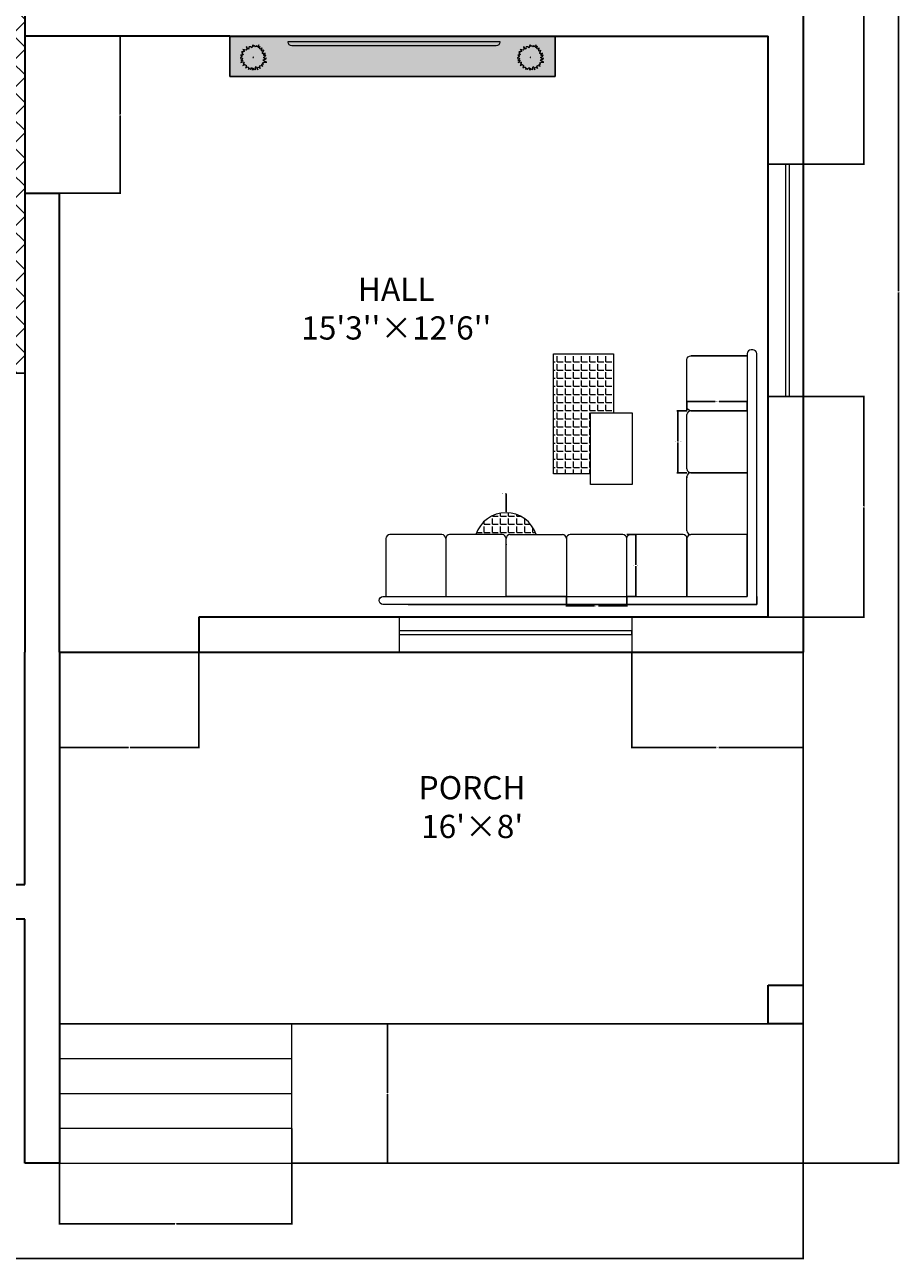
# Model space of a CAD drawing. Units: inches. Extents: x 1315 to 1802, y 1702 to 2202.
# Tile 3 of 4: x 1577 to 1802, y 1702 to 2021. Entities that reach past the tile are written whole.
import ezdxf

# ---------------------------------------------------------------- set-up
doc = ezdxf.new("R2010")
doc.units = ezdxf.units.IN
for name, color, linetype, lineweight in [('A-ANNO-DIMS', 2, 'Continuous', 18), ('A-AREA-IDEN', 3, 'Continuous', 18), ('A-CASE', 7, 'Continuous', 25), ('A-CASE-PATT', 246, 'Continuous', 13), ('A-COLS', 7, 'Continuous', 35), ('A-EQPM', 3, 'Continuous', 18), ('A-FLOR', 7, 'Continuous', 25), ('A-FLOR-PATT', 254, 'Continuous', 13), ('A-FLOR-STRS', 7, 'Continuous', 18), ('A-FURN', 8, 'Continuous', 18), ('A-FURN-PATT', 9, 'Continuous', 13), ('A-GLAZ', 4, 'Continuous', 18), ('A-WALL', 7, 'Continuous', 35)]:
    doc.layers.add(name, color=color, linetype=linetype, lineweight=lineweight)
doc.styles.get("Standard").update_dxf_attribs({"font": 'times.ttf'})
doc.dimstyles.get("Standard").update_dxf_attribs({"dimtxt": 0.18, "dimasz": 0.18, "dimexe": 0.18, "dimexo": 0.0625, "dimgap": 0.09, "dimtad": 0, "dimtih": 1, "dimtoh": 1, "dimdec": 4, "dimzin": 0, "dimdsep": 46, "dimtxsty": 'Standard', "dimcen": 0.09, "dimadec": 0, "dimazin": 0, "dimtfac": 1, "dimtdec": 4, "dimtofl": 0, "dimtmove": 0, "dimatfit": 3, "dimfxl": 1, "dimtolj": 1, "dimtzin": 0, "dimarcsym": 0})

# ---------------------------------------------------------------- blocks, each defined once
blk = doc.blocks.new('*U2')
for points in [[(0, 60.64), (-3.051, 56.238), (-4.196, 52.815), (-5.34, 47.925), (-6.103, 45.969), (-11.062, 50.859), (-18.691, 52.326), (-20.98, 47.436), (-20.217, 43.524), (-20.598, 39.611), (-25.939, 43.035), (-27.846, 49.392), (-33.186, 52.326), (-30.516, 47.436), (-31.279, 43.035), (-30.135, 38.144), (-33.568, 35.21), (-40.815, 36.677), (-49.208, 38.144), (-46.919, 36.677), (-42.341, 31.787), (-42.341, 28.364), (-46.537, 27.386), (-55.692, 27.386), (-49.97, 22.006), (-54.548, 21.028), (-46.156, 14.671), (-51.496, 11.248), (-59.888, 11.248), (-55.692, 8.803), (-53.785, 5.38), (-57.218, 3.423), (-60.651, -1.467), (-61.033, -4.89), (-59.125, -3.423), (-54.548, -1.467), (-51.496, -4.401), (-53.022, -10.269), (-59.125, -15.16), (-49.208, -13.204), (-58.362, -24.451), (-48.445, -21.028), (-43.486, -22.495), (-43.104, -25.918), (-47.3, -31.298), (-43.104, -30.32), (-48.445, -39.611), (-38.527, -31.787), (-40.815, -36.188), (-32.423, -37.166), (-33.568, -43.523), (-35.475, -49.392), (-28.609, -44.99), (-23.65, -46.457), (-22.124, -51.837), (-21.743, -57.705), (-19.073, -52.326), (-15.639, -51.837), (-12.588, -58.683), (-11.062, -54.771), (-6.866, -49.392), (-6.866, -53.304), (-4.959, -48.414), (-1.907, -61.617), (-1.144, -51.348), (4.578, -59.172), (5.341, -54.282), (9.918, -56.727), (12.207, -60.639), (12.97, -47.925), (14.877, -44.501), (17.547, -47.436), (19.455, -52.815), (22.888, -60.639), (21.743, -49.392), (23.65, -46.457), (29.754, -47.925), (35.094, -52.326), (37.001, -53.793), (33.187, -46.457), (32.042, -41.567), (35.094, -39.122), (43.868, -40.589), (47.682, -42.056), (43.105, -36.188), (43.105, -33.743), (46.538, -31.298), (50.352, -32.765), (46.919, -26.407), (55.693, -22.495), (60.652, -22.984), (66.374, -22.006), (59.889, -20.05), (54.167, -18.094), (51.878, -15.649), (49.589, -12.225), (51.497, -10.269), (57.981, -9.78), (63.322, -7.335), (64.466, -2.934)], [(64.848, -2.934), (59.507, -5.379), (56.456, -4.401), (51.878, -2.445), (52.26, 0.978), (55.311, 3.912), (59.889, 5.869), (62.94, 11.248), (58.363, 10.27), (54.548, 10.27), (51.115, 11.248), (53.785, 15.649), (57.981, 18.094), (60.652, 19.561), (56.074, 19.561), (51.115, 17.605), (46.538, 19.072), (46.156, 22.496), (49.589, 27.386), (52.26, 34.721), (49.589, 33.743), (44.249, 30.32), (41.197, 32.276), (41.579, 37.655), (43.868, 42.546), (43.105, 46.947), (40.053, 44.013), (36.238, 40.589), (33.568, 42.057), (33.95, 45.969), (35.476, 52.815), (31.28, 49.392), (26.702, 46.947), (28.228, 50.859), (28.609, 61.129), (24.795, 54.282), (18.692, 50.859), (17.929, 57.706), (12.97, 50.859), (7.248, 57.706), (5.341, 53.304), (0, 60.64)]]:
    blk.add_lwpolyline(points)
blk.add_lwpolyline([(0.382, 1.956), (0, 0), (1.907, 0.489), (2.289, 1.467)], close=True)
blk = doc.blocks.new('SEFVFT')
for p, q in [((1768.59, 1985.26), (1777.59, 1985.26)), ((1768.59, 1925.26), (1768.59, 1985.26)), ((1768.59, 1985.26), (1773.09, 1985.26)), ((1773.09, 1985.26), (1773.09, 1925.26)), ((1774.09, 1925.26), (1774.09, 1985.26)), ((1777.59, 1985.26), (1777.59, 1925.26)), ((1777.59, 1925.26), (1768.59, 1925.26)), ((1773.09, 1925.26), (1774.09, 1925.26))]:
    blk.add_line(p, q)
blk = doc.blocks.new('SOFA-SEAT')
for p, q in [((14.58, 16), (1, 16)), ((0, 15), (0, 0)), ((15.58, 0), (15.58, 15)), ((0, 0), (15.58, 0))]:
    blk.add_line(p, q)
for centre, start, end in [((1, 15), 90, 180), ((14.58, 15), 0, 90)]:
    blk.add_arc(centre, 1, start, end)
blk = doc.blocks.new('SOFA-RETURN-SEAT')
for p, q in [((1, 16), (15.58, 16)), ((15.58, 16), (15.58, 0)), ((0, 1), (0, 15)), ((15.58, 0), (1, 0))]:
    blk.add_line(p, q)
for centre, start, end in [((1, 15), 90, 180), ((1, 1), 180, 270)]:
    blk.add_arc(centre, 1, start, end)
blk = doc.blocks.new('*D24')
at = {"layer": 'A-ANNO-DIMS', "color": 0, "lineweight": -2, "transparency": 16777216}
for p, q in [((1732.1, 1889.55), (1734.62, 1889.55)), ((1734.44, 1889.37), (1734.44, 1881.73)), ((1734.44, 1873.73), (1734.44, 1881.37)), ((1732.1, 1873.55), (1734.62, 1873.55))]:
    blk.add_line(p, q, dxfattribs=at)
at = {"layer": 'A-ANNO-DIMS', "color": 0, "transparency": 16777216}
for points in [[(1734.41, 1889.37), (1734.47, 1889.37), (1734.44, 1889.55)], [(1734.41, 1873.73), (1734.47, 1873.73), (1734.44, 1873.55)]]:
    blk.add_solid(points, dxfattribs=at)
at = {"layer": 'Defpoints', "color": 0, "transparency": 16777216}
for p in [(1732.04, 1889.55), (1734.44, 1889.55), (1732.04, 1873.55)]:
    blk.add_point(p, dxfattribs=at)
at = {"layer": 'A-ANNO-DIMS', "color": 0, "transparency": 16777216, "insert": (1734.44, 1881.55), "char_height": 0.18, "attachment_point": 5}
blk.add_mtext('\\A1;SEAT 16 TYP.', dxfattribs=at)
blk = doc.blocks.new('*D25')
at = {"layer": 'A-ANNO-DIMS', "color": 0, "lineweight": -2, "transparency": 16777216}
for p, q in [((1716.46, 1873.49), (1716.46, 1870.97)), ((1732.04, 1873.49), (1732.04, 1870.97)), ((1716.64, 1871.15), (1723.74, 1871.15)), ((1731.86, 1871.15), (1724.77, 1871.15))]:
    blk.add_line(p, q, dxfattribs=at)
at = {"layer": 'A-ANNO-DIMS', "color": 0, "transparency": 16777216}
for points in [[(1716.64, 1871.18), (1716.64, 1871.12), (1716.46, 1871.15)], [(1731.86, 1871.18), (1731.86, 1871.12), (1732.04, 1871.15)]]:
    blk.add_solid(points, dxfattribs=at)
at = {"layer": 'Defpoints', "color": 0, "transparency": 16777216}
for p in [(1716.46, 1873.55), (1732.04, 1873.55), (1732.04, 1871.15)]:
    blk.add_point(p, dxfattribs=at)
at = {"layer": 'A-ANNO-DIMS', "color": 0, "transparency": 16777216, "insert": (1724.25, 1871.15), "char_height": 0.18, "attachment_point": 5}
blk.add_mtext('\\A1;16 TYP.', dxfattribs=at)
blk = doc.blocks.new('*D26')
at = {"layer": 'A-ANNO-DIMS', "color": 0, "lineweight": -2, "transparency": 16777216}
for p, q in [((1747.55, 1921.54), (1745.03, 1921.54)), ((1745.21, 1921.36), (1745.21, 1913.73)), ((1745.21, 1905.73), (1745.21, 1913.36)), ((1747.55, 1905.55), (1745.03, 1905.55))]:
    blk.add_line(p, q, dxfattribs=at)
at = {"layer": 'A-ANNO-DIMS', "color": 0, "transparency": 16777216}
for points in [[(1745.18, 1921.36), (1745.24, 1921.36), (1745.21, 1921.54)], [(1745.18, 1905.73), (1745.24, 1905.73), (1745.21, 1905.55)]]:
    blk.add_solid(points, dxfattribs=at)
at = {"layer": 'Defpoints', "color": 0, "transparency": 16777216}
for p in [(1745.21, 1921.54), (1747.61, 1921.54), (1747.61, 1905.55)]:
    blk.add_point(p, dxfattribs=at)
at = {"layer": 'A-ANNO-DIMS', "color": 0, "transparency": 16777216, "insert": (1745.21, 1913.55), "char_height": 0.18, "attachment_point": 5}
blk.add_mtext('\\A1;RETURN SEAT 16 TYP.', dxfattribs=at)
blk = doc.blocks.new('*D27')
at = {"layer": 'A-ANNO-DIMS', "color": 0, "lineweight": -2, "transparency": 16777216}
for p, q in [((1747.61, 1921.61), (1747.61, 1924.12)), ((1747.79, 1923.94), (1754.89, 1923.94)), ((1763.01, 1923.94), (1755.92, 1923.94)), ((1763.19, 1921.61), (1763.19, 1924.12))]:
    blk.add_line(p, q, dxfattribs=at)
at = {"layer": 'A-ANNO-DIMS', "color": 0, "transparency": 16777216}
for points in [[(1747.79, 1923.97), (1747.79, 1923.91), (1747.61, 1923.94)], [(1763.01, 1923.97), (1763.01, 1923.91), (1763.19, 1923.94)]]:
    blk.add_solid(points, dxfattribs=at)
at = {"layer": 'Defpoints', "color": 0, "transparency": 16777216}
for p in [(1763.19, 1923.94), (1747.61, 1921.54), (1763.19, 1921.54)]:
    blk.add_point(p, dxfattribs=at)
at = {"layer": 'A-ANNO-DIMS', "color": 0, "transparency": 16777216, "insert": (1755.4, 1923.94), "char_height": 0.18, "attachment_point": 5}
blk.add_mtext('\\A1;16 TYP.', dxfattribs=at)
blk = doc.blocks.new('*D28')
at = {"layer": 'A-ANNO-DIMS', "color": 0, "lineweight": -2, "transparency": 16777216}
for p, q in [((1339.59, 1931.18), (1339.59, 1702.41)), ((1777.59, 1763.18), (1777.59, 1702.41)), ((1339.77, 1702.59), (1558.31, 1702.59)), ((1777.41, 1702.59), (1558.87, 1702.59))]:
    blk.add_line(p, q, dxfattribs=at)
at = {"layer": 'A-ANNO-DIMS', "color": 0, "transparency": 16777216}
for points in [[(1339.77, 1702.62), (1339.77, 1702.56), (1339.59, 1702.59)], [(1777.41, 1702.62), (1777.41, 1702.56), (1777.59, 1702.59)]]:
    blk.add_solid(points, dxfattribs=at)
at = {"layer": 'Defpoints', "color": 0, "transparency": 16777216}
for p in [(1339.59, 1931.24), (1777.59, 1763.24), (1777.59, 1702.59)]:
    blk.add_point(p, dxfattribs=at)
at = {"layer": 'A-ANNO-DIMS', "color": 0, "transparency": 16777216, "insert": (1558.59, 1702.59), "char_height": 0.18, "attachment_point": 5}
blk.add_mtext('\\A1;438', dxfattribs=at)
blk = doc.blocks.new('*D29')
at = {"layer": 'A-ANNO-DIMS', "color": 0, "lineweight": -2, "transparency": 16777216}
for p, q in [((1777.65, 2177.24), (1802.42, 2177.24)), ((1802.24, 2177.06), (1802.24, 1952.42)), ((1802.24, 1727.42), (1802.24, 1952.06)), ((1645.65, 1727.24), (1802.42, 1727.24))]:
    blk.add_line(p, q, dxfattribs=at)
at = {"layer": 'A-ANNO-DIMS', "color": 0, "transparency": 16777216}
for points in [[(1802.21, 2177.06), (1802.27, 2177.06), (1802.24, 2177.24)], [(1802.21, 1727.42), (1802.27, 1727.42), (1802.24, 1727.24)]]:
    blk.add_solid(points, dxfattribs=at)
at = {"layer": 'Defpoints', "color": 0, "transparency": 16777216}
for p in [(1777.59, 2177.24), (1802.24, 2177.24), (1645.59, 1727.24)]:
    blk.add_point(p, dxfattribs=at)
at = {"layer": 'A-ANNO-DIMS', "color": 0, "transparency": 16777216, "insert": (1802.24, 1952.24), "char_height": 0.18, "attachment_point": 5}
blk.add_mtext('\\A1;450', dxfattribs=at)
blk = doc.blocks.new('*D42')
at = {"layer": 'A-ANNO-DIMS', "color": 0, "lineweight": -2, "transparency": 16777216}
for p, q in [((1768.65, 2072.19), (1793.42, 2072.19)), ((1793.24, 2072.01), (1793.24, 2028.91)), ((1793.24, 1985.44), (1793.24, 2028.54)), ((1768.65, 1985.26), (1793.42, 1985.26))]:
    blk.add_line(p, q, dxfattribs=at)
at = {"layer": 'A-ANNO-DIMS', "color": 0, "transparency": 16777216}
for points in [[(1793.21, 2072.01), (1793.27, 2072.01), (1793.24, 2072.19)], [(1793.21, 1985.44), (1793.27, 1985.44), (1793.24, 1985.26)]]:
    blk.add_solid(points, dxfattribs=at)
at = {"layer": 'Defpoints', "color": 0, "transparency": 16777216}
for p in [(1768.59, 2072.19), (1768.59, 1985.26), (1793.24, 1985.26)]:
    blk.add_point(p, dxfattribs=at)
at = {"layer": 'A-ANNO-DIMS', "color": 0, "transparency": 16777216, "insert": (1793.24, 2028.72), "char_height": 0.18, "attachment_point": 5}
blk.add_mtext('\\A1;86.94', dxfattribs=at)
blk = doc.blocks.new('*D43')
at = {"layer": 'A-ANNO-DIMS', "color": 0, "lineweight": -2, "transparency": 16777216}
for p, q in [((1768.65, 1925.26), (1793.42, 1925.26)), ((1793.24, 1925.08), (1793.24, 1896.93)), ((1793.24, 1868.42), (1793.24, 1896.57)), ((1768.65, 1868.24), (1793.42, 1868.24))]:
    blk.add_line(p, q, dxfattribs=at)
at = {"layer": 'A-ANNO-DIMS', "color": 0, "transparency": 16777216}
for points in [[(1793.21, 1925.08), (1793.27, 1925.08), (1793.24, 1925.26)], [(1793.21, 1868.42), (1793.27, 1868.42), (1793.24, 1868.24)]]:
    blk.add_solid(points, dxfattribs=at)
at = {"layer": 'Defpoints', "color": 0, "transparency": 16777216}
for p in [(1768.59, 1925.26), (1768.59, 1868.24), (1793.24, 1868.24)]:
    blk.add_point(p, dxfattribs=at)
at = {"layer": 'A-ANNO-DIMS', "color": 0, "transparency": 16777216, "insert": (1793.24, 1896.75), "char_height": 0.18, "attachment_point": 5}
blk.add_mtext('\\A1;57.01', dxfattribs=at)
blk = doc.blocks.new('*D44')
at = {"layer": 'A-ANNO-DIMS', "color": 0, "lineweight": -2, "transparency": 16777216}
for p, q in [((1645.65, 1763.24), (1670.42, 1763.24)), ((1670.24, 1763.06), (1670.24, 1745.42)), ((1670.24, 1727.42), (1670.24, 1745.06)), ((1645.65, 1727.24), (1670.42, 1727.24))]:
    blk.add_line(p, q, dxfattribs=at)
at = {"layer": 'A-ANNO-DIMS', "color": 0, "transparency": 16777216}
for points in [[(1670.21, 1763.06), (1670.27, 1763.06), (1670.24, 1763.24)], [(1670.21, 1727.42), (1670.27, 1727.42), (1670.24, 1727.24)]]:
    blk.add_solid(points, dxfattribs=at)
at = {"layer": 'Defpoints', "color": 0, "transparency": 16777216}
for p in [(1645.59, 1763.24), (1645.59, 1727.24), (1670.24, 1727.24)]:
    blk.add_point(p, dxfattribs=at)
at = {"layer": 'A-ANNO-DIMS', "color": 0, "transparency": 16777216, "insert": (1670.24, 1745.24), "char_height": 0.18, "attachment_point": 5}
blk.add_mtext('\\A1;36', dxfattribs=at)
blk = doc.blocks.new('*D47')
at = {"layer": 'A-ANNO-DIMS', "color": 0, "lineweight": -2, "transparency": 16777216}
for p, q in [((1585.59, 1736.18), (1585.59, 1711.41)), ((1645.59, 1736.18), (1645.59, 1711.41)), ((1585.77, 1711.59), (1615.38, 1711.59)), ((1645.41, 1711.59), (1615.8, 1711.59))]:
    blk.add_line(p, q, dxfattribs=at)
at = {"layer": 'A-ANNO-DIMS', "color": 0, "transparency": 16777216}
for points in [[(1585.77, 1711.62), (1585.77, 1711.56), (1585.59, 1711.59)], [(1645.41, 1711.62), (1645.41, 1711.56), (1645.59, 1711.59)]]:
    blk.add_solid(points, dxfattribs=at)
at = {"layer": 'Defpoints', "color": 0, "transparency": 16777216}
for p in [(1585.59, 1736.24), (1645.59, 1736.24), (1585.59, 1711.59)]:
    blk.add_point(p, dxfattribs=at)
at = {"layer": 'A-ANNO-DIMS', "color": 0, "transparency": 16777216, "insert": (1615.59, 1711.59), "char_height": 0.18, "attachment_point": 5}
blk.add_mtext('\\A1;60', dxfattribs=at)
blk = doc.blocks.new('*D48')
at = {"layer": 'A-ANNO-DIMS', "color": 0, "lineweight": -2, "transparency": 16777216}
for p, q in [((1733.38, 1859.18), (1733.38, 1834.41)), ((1777.59, 1859.18), (1777.59, 1834.41)), ((1733.56, 1834.59), (1755.11, 1834.59)), ((1777.41, 1834.59), (1755.85, 1834.59))]:
    blk.add_line(p, q, dxfattribs=at)
at = {"layer": 'A-ANNO-DIMS', "color": 0, "transparency": 16777216}
for points in [[(1733.56, 1834.62), (1733.56, 1834.56), (1733.38, 1834.59)], [(1777.41, 1834.62), (1777.41, 1834.56), (1777.59, 1834.59)]]:
    blk.add_solid(points, dxfattribs=at)
at = {"layer": 'Defpoints', "color": 0, "transparency": 16777216}
for p in [(1733.38, 1859.24), (1777.59, 1859.24), (1733.38, 1834.59)]:
    blk.add_point(p, dxfattribs=at)
at = {"layer": 'A-ANNO-DIMS', "color": 0, "transparency": 16777216, "insert": (1755.48, 1834.59), "char_height": 0.18, "attachment_point": 5}
blk.add_mtext('\\A1;44.21', dxfattribs=at)
blk = doc.blocks.new('*D52')
at = {"layer": 'A-ANNO-DIMS', "color": 0, "lineweight": -2, "transparency": 16777216}
for p, q in [((1576.65, 2018.24), (1601.42, 2018.24)), ((1601.24, 2018.06), (1601.24, 1998.17)), ((1601.24, 1977.92), (1601.24, 1997.81)), ((1576.65, 1977.74), (1601.42, 1977.74))]:
    blk.add_line(p, q, dxfattribs=at)
at = {"layer": 'A-ANNO-DIMS', "color": 0, "transparency": 16777216}
for points in [[(1601.21, 2018.06), (1601.27, 2018.06), (1601.24, 2018.24)], [(1601.21, 1977.92), (1601.27, 1977.92), (1601.24, 1977.74)]]:
    blk.add_solid(points, dxfattribs=at)
at = {"layer": 'Defpoints', "color": 0, "transparency": 16777216}
for p in [(1576.59, 2018.24), (1576.59, 1977.74), (1601.24, 1977.74)]:
    blk.add_point(p, dxfattribs=at)
at = {"layer": 'A-ANNO-DIMS', "color": 0, "transparency": 16777216, "insert": (1601.24, 1997.99), "char_height": 0.18, "attachment_point": 5}
blk.add_mtext('\\A1;40.5', dxfattribs=at)
blk = doc.blocks.new('*D54')
at = {"layer": 'A-ANNO-DIMS', "color": 0, "lineweight": -2, "transparency": 16777216}
for p, q in [((1585.59, 1859.18), (1585.59, 1834.41)), ((1621.59, 1859.18), (1621.59, 1834.41)), ((1585.77, 1834.59), (1603.38, 1834.59)), ((1621.41, 1834.59), (1603.8, 1834.59))]:
    blk.add_line(p, q, dxfattribs=at)
at = {"layer": 'A-ANNO-DIMS', "color": 0, "transparency": 16777216}
for points in [[(1585.77, 1834.62), (1585.77, 1834.56), (1585.59, 1834.59)], [(1621.41, 1834.62), (1621.41, 1834.56), (1621.59, 1834.59)]]:
    blk.add_solid(points, dxfattribs=at)
at = {"layer": 'Defpoints', "color": 0, "transparency": 16777216}
for p in [(1585.59, 1859.24), (1621.59, 1859.24), (1585.59, 1834.59)]:
    blk.add_point(p, dxfattribs=at)
at = {"layer": 'A-ANNO-DIMS', "color": 0, "transparency": 16777216, "insert": (1603.59, 1834.59), "char_height": 0.18, "attachment_point": 5}
blk.add_mtext('\\A1;36', dxfattribs=at)
blk = doc.blocks.new('*D60')
at = {"layer": 'A-ANNO-DIMS', "color": 0, "lineweight": -2, "transparency": 16777216}
for p, q in [((1700.71, 1900.13), (1700.89, 1900.13)), ((1700.89, 1900.13), (1700.89, 1895.4)), ((1700.8, 1887.04), (1700.98, 1887.04)), ((1700.89, 1886.95), (1700.89, 1887.13))]:
    blk.add_line(p, q, dxfattribs=at)
at = {"layer": 'A-ANNO-DIMS', "color": 0, "transparency": 16777216}
blk.add_solid([(1700.92, 1895.4), (1700.86, 1895.4), (1700.89, 1895.22)], dxfattribs=at)
at = {"layer": 'Defpoints', "color": 0, "transparency": 16777216}
for p in [(1700.89, 1895.22), (1700.89, 1887.04)]:
    blk.add_point(p, dxfattribs=at)
at = {"layer": 'A-ANNO-DIMS', "color": 0, "transparency": 16777216, "insert": (1700.24, 1900.13), "char_height": 0.18, "attachment_point": 5}
blk.add_mtext('\\A1;R8.182', dxfattribs=at)

msp = doc.modelspace()

# ---------------------------------------------------------------- hatches: boundary and pattern name
at = {"layer": 'A-CASE-PATT'}
h = msp.add_hatch(color=256, dxfattribs=at)
h.dxf.hatch_style = 1
h.paths.add_polyline_path([(1713.5889, 2018.2411), (1629.5889, 2018.2411), (1629.5889, 2007.8552), (1713.5889, 2007.8552)])
h.paths.add_polyline_path([(1645.5983, 2015.7518, -0.41421356), (1644.5983, 2016.7518), (1644.5983, 2016.9053), (1699.2987, 2016.9053), (1699.2987, 2016.7518, -0.41421356), (1698.2987, 2015.7518)], flags=16)
h.paths.add_polyline_path([(1703.8701, 2012.5137), (1703.8904, 2012.6962), (1704.0735, 2012.957), (1704.2565, 2013.0613), (1704.1548, 2013.2438), (1703.9311, 2013.3742), (1704.3785, 2013.3742), (1704.6633, 2013.5567), (1704.2158, 2013.8956), (1704.4599, 2013.9477), (1704.1548, 2014.2346), (1704.6429, 2014.2346), (1704.8667, 2014.2867), (1704.8667, 2014.4692), (1704.6226, 2014.73), (1704.5005, 2014.8082), (1704.948, 2014.73), (1705.3344, 2014.6517), (1705.5174, 2014.8082), (1705.4565, 2015.0689), (1705.4971, 2015.3036), (1705.3548, 2015.5643), (1705.6395, 2015.4079), (1705.7412, 2015.0689), (1706.0259, 2014.8864), (1706.0462, 2015.095), (1706.0056, 2015.3036), (1706.1276, 2015.5643), (1706.5344, 2015.4861), (1706.7988, 2015.2254), (1706.8394, 2015.3297), (1706.9004, 2015.5904), (1706.9615, 2015.7729), (1707.1241, 2016.0076), (1707.4089, 2015.6165), (1707.5106, 2015.8512), (1707.8157, 2015.4861), (1708.0801, 2015.8512), (1708.1207, 2015.4861), (1708.4461, 2015.6686), (1708.6495, 2016.0337), (1708.6292, 2015.4861), (1708.5478, 2015.2775), (1708.7919, 2015.4079), (1709.0156, 2015.5904), (1708.9342, 2015.2254), (1708.9139, 2015.0168), (1709.0562, 2014.9385), (1709.2596, 2015.1211), (1709.4224, 2015.2775), (1709.463, 2015.0429), (1709.341, 2014.7821), (1709.3206, 2014.4953), (1709.4834, 2014.391), (1709.7681, 2014.5735), (1709.9105, 2014.6257), (1709.7681, 2014.2346), (1709.585, 2013.9739), (1709.6054, 2013.7913), (1709.8494, 2013.7131), (1710.1138, 2013.8174), (1710.3579, 2013.8174), (1710.2155, 2013.7392), (1709.9918, 2013.6088), (1709.8494, 2013.3742), (1710.0325, 2013.322), (1710.2359, 2013.322), (1710.4799, 2013.3742), (1710.3172, 2013.0874), (1710.0731, 2012.983), (1709.9105, 2012.8266), (1709.8901, 2012.6441), (1710.1342, 2012.5398), (1710.2969, 2012.4877), (1710.5585, 2012.6074), (1710.5003, 2012.3834), (1710.2155, 2012.253), (1709.8698, 2012.2269), (1709.7681, 2012.1227), (1709.8901, 2011.9401), (1710.0122, 2011.8097), (1710.3172, 2011.7055), (1710.663, 2011.6012), (1710.3579, 2011.549), (1710.0935, 2011.5751), (1709.6257, 2011.3665), (1709.8087, 2011.0275), (1709.6054, 2011.1057), (1709.4224, 2010.9754), (1709.4224, 2010.845), (1709.6664, 2010.5322), (1709.463, 2010.6104), (1708.9952, 2010.6886), (1708.8325, 2010.5582), (1708.8936, 2010.2975), (1709.0969, 2009.9064), (1708.9952, 2009.9846), (1708.7105, 2010.2193), (1708.3851, 2010.2975), (1708.2834, 2010.141), (1708.3445, 2009.5414), (1708.1614, 2009.9585), (1708.0597, 2010.2453), (1707.9173, 2010.4018), (1707.8157, 2010.2193), (1707.775, 2009.5414), (1707.6529, 2009.75), (1707.4089, 2009.8803), (1707.3682, 2009.6196), (1707.0632, 2010.0367), (1707.0225, 2009.4892), (1706.8597, 2010.1932), (1706.7581, 2009.9325), (1706.7581, 2010.141), (1706.5344, 2009.8542), (1706.453, 2009.6457), (1706.2903, 2010.0107), (1706.1072, 2009.9846), (1705.9649, 2009.6978), (1705.9446, 2010.0107), (1705.8632, 2010.2975), (1705.5988, 2010.3757), (1705.2327, 2010.141), (1705.3344, 2010.454), (1705.3955, 2010.7929), (1704.948, 2010.845), (1705.07, 2011.0797), (1704.5412, 2010.6625), (1704.826, 2011.1579), (1704.6023, 2011.1057), (1704.826, 2011.3926), (1704.8056, 2011.5751), (1704.5412, 2011.6533), (1704.0125, 2011.4708), (1704.5005, 2012.0705), (1703.9718, 2011.9662), (1704.2972, 2012.2269), (1704.3785, 2012.5398), (1704.2158, 2012.6962), (1703.9718, 2012.592)], flags=16)
h.paths.add_polyline_path([(1707.1241, 2012.7745), (1707.1445, 2012.8787), (1707.2462, 2012.8527), (1707.2258, 2012.8005)], flags=0)
h.paths.add_polyline_path([(1639.0758, 2011.6012), (1638.7707, 2011.549), (1638.5063, 2011.5751), (1638.0385, 2011.3665), (1638.2216, 2011.0275), (1638.0182, 2011.1057), (1637.8352, 2010.9754), (1637.8352, 2010.845), (1638.0792, 2010.5322), (1637.8759, 2010.6104), (1637.408, 2010.6886), (1637.2453, 2010.5582), (1637.3064, 2010.2975), (1637.5097, 2009.9064), (1637.408, 2009.9846), (1637.1233, 2010.2193), (1636.7979, 2010.2975), (1636.6962, 2010.141), (1636.7573, 2009.5414), (1636.5742, 2009.9585), (1636.4725, 2010.2453), (1636.3301, 2010.4018), (1636.2285, 2010.2193), (1636.1878, 2009.5414), (1636.0657, 2009.75), (1635.8217, 2009.8803), (1635.781, 2009.6196), (1635.476, 2010.0367), (1635.4353, 2009.4892), (1635.2726, 2010.1932), (1635.1709, 2009.9325), (1635.1709, 2010.141), (1634.9472, 2009.8542), (1634.8658, 2009.6457), (1634.7031, 2010.0107), (1634.52, 2009.9846), (1634.3777, 2009.6978), (1634.3574, 2010.0107), (1634.276, 2010.2975), (1634.0116, 2010.3757), (1633.6455, 2010.141), (1633.7472, 2010.454), (1633.8083, 2010.7929), (1633.3608, 2010.845), (1633.4828, 2011.0797), (1632.954, 2010.6625), (1633.2388, 2011.1579), (1633.0151, 2011.1057), (1633.2388, 2011.3926), (1633.2184, 2011.5751), (1632.954, 2011.6533), (1632.4253, 2011.4708), (1632.9133, 2012.0705), (1632.3846, 2011.9662), (1632.71, 2012.2269), (1632.7914, 2012.5398), (1632.6286, 2012.6962), (1632.3846, 2012.592), (1632.2829, 2012.5137), (1632.3032, 2012.6962), (1632.4863, 2012.957), (1632.6693, 2013.0613), (1632.5676, 2013.2438), (1632.3439, 2013.3742), (1632.7914, 2013.3742), (1633.0761, 2013.5567), (1632.6286, 2013.8956), (1632.8727, 2013.9477), (1632.5676, 2014.2346), (1633.0558, 2014.2346), (1633.2795, 2014.2867), (1633.2795, 2014.4692), (1633.0354, 2014.73), (1632.9133, 2014.8082), (1633.3608, 2014.73), (1633.7472, 2014.6517), (1633.9303, 2014.8082), (1633.8693, 2015.0689), (1633.9099, 2015.3036), (1633.7676, 2015.5643), (1634.0523, 2015.4079), (1634.154, 2015.0689), (1634.4387, 2014.8864), (1634.459, 2015.095), (1634.4184, 2015.3036), (1634.5404, 2015.5643), (1634.9472, 2015.4861), (1635.2116, 2015.2254), (1635.2522, 2015.3297), (1635.3132, 2015.5904), (1635.3743, 2015.7729), (1635.537, 2016.0076), (1635.8217, 2015.6165), (1635.9234, 2015.8512), (1636.2285, 2015.4861), (1636.4929, 2015.8512), (1636.5335, 2015.4861), (1636.8589, 2015.6686), (1637.0623, 2016.0337), (1637.042, 2015.4861), (1636.9606, 2015.2775), (1637.2047, 2015.4079), (1637.4284, 2015.5904), (1637.3471, 2015.2254), (1637.3267, 2015.0168), (1637.469, 2014.9385), (1637.6724, 2015.1211), (1637.8352, 2015.2775), (1637.8759, 2015.0429), (1637.7538, 2014.7821), (1637.7334, 2014.4953), (1637.8962, 2014.391), (1638.1809, 2014.5735), (1638.3233, 2014.6257), (1638.1809, 2014.2346), (1637.9978, 2013.9739), (1638.0182, 2013.7913), (1638.2622, 2013.7131), (1638.5266, 2013.8174), (1638.7707, 2013.8174), (1638.6283, 2013.7392), (1638.4046, 2013.6088), (1638.2622, 2013.3742), (1638.4453, 2013.322), (1638.6487, 2013.322), (1638.8927, 2013.3742), (1638.73, 2013.0874), (1638.486, 2012.983), (1638.3233, 2012.8266), (1638.3029, 2012.6441), (1638.547, 2012.5398), (1638.7097, 2012.4877), (1638.9713, 2012.6074), (1638.9131, 2012.3834), (1638.6283, 2012.253), (1638.2826, 2012.2269), (1638.1809, 2012.1227), (1638.3029, 2011.9401), (1638.425, 2011.8097), (1638.73, 2011.7055)], flags=16)
h.paths.add_polyline_path([(1635.659, 2012.8527), (1635.6386, 2012.8005), (1635.537, 2012.7745), (1635.5573, 2012.8787)], flags=0)
at = {"layer": 'A-FLOR-PATT'}
h = msp.add_hatch(dxfattribs=at)
h.set_pattern_fill('AR-HBONE', color=256, scale=0.05)
h.paths.add_polyline_path([(1576.5889, 2024.2411), (1629.5889, 2024.2411), (1629.5889, 2060.2411), (1629.5889, 2113.2411), (1587.5889, 2113.2411), (1587.5889, 2077.2411), (1532.5889, 2077.2411), (1532.5889, 2015.2411), (1532.5889, 1931.2411), (1576.5889, 1931.2411), (1576.5889, 1940.2411)])
h.paths.add_polyline_path([(1533.7746, 2061.9724), (1533.7746, 2075.958), (1570.2638, 2075.958), (1570.2638, 2061.9724)], flags=16)
edge = h.paths.add_edge_path(flags=0)
edge.add_ellipse((1551.6328, 2068.3646), major_axis=(-10.9397, 0), ratio=0.44313735, start_angle=273.23456, end_angle=623.06073, ccw=False)
edge.add_line((1551.359, 2073.2109), (1551.359, 2073.9173))
edge.add_line((1551.359, 2073.9173), (1552.222, 2073.9173))
edge.add_line((1552.222, 2073.9173), (1552.222, 2073.2053))
h.paths.add_polyline_path([(1551.0754, 2068.4287, -1), (1552.5545, 2068.4287, -1)], flags=0)
at = {"layer": 'A-FURN-PATT'}
h = msp.add_hatch(color=256, dxfattribs=at)
h.dxf.hatch_style = 1
h.paths.add_polyline_path([(1637.8759, 2010.6104), (1638.0792, 2010.5322), (1637.8352, 2010.845), (1637.8352, 2010.9754), (1638.0182, 2011.1057), (1638.2216, 2011.0275), (1638.0385, 2011.3665), (1638.5063, 2011.5751), (1638.7707, 2011.549), (1639.0758, 2011.6012), (1638.73, 2011.7055), (1638.425, 2011.8097), (1638.3029, 2011.9401), (1638.1809, 2012.1227), (1638.2826, 2012.2269), (1638.6283, 2012.253), (1638.9131, 2012.3834), (1638.9713, 2012.6074), (1638.7097, 2012.4877), (1638.547, 2012.5398), (1638.3029, 2012.6441), (1638.3233, 2012.8266), (1638.486, 2012.983), (1638.73, 2013.0874), (1638.8927, 2013.3742), (1638.6487, 2013.322), (1638.4453, 2013.322), (1638.2622, 2013.3742), (1638.4046, 2013.6088), (1638.6283, 2013.7392), (1638.7707, 2013.8174), (1638.5266, 2013.8174), (1638.2622, 2013.7131), (1638.0182, 2013.7913), (1637.9978, 2013.9739), (1638.1809, 2014.2346), (1638.3233, 2014.6257), (1638.1809, 2014.5735), (1637.8962, 2014.391), (1637.7334, 2014.4953), (1637.7538, 2014.7821), (1637.8759, 2015.0429), (1637.8352, 2015.2775), (1637.6724, 2015.1211), (1637.469, 2014.9385), (1637.3267, 2015.0168), (1637.3471, 2015.2254), (1637.4284, 2015.5904), (1637.2047, 2015.4079), (1636.9606, 2015.2775), (1637.042, 2015.4861), (1637.0623, 2016.0337), (1636.8589, 2015.6686), (1636.5335, 2015.4861), (1636.4929, 2015.8512), (1636.2285, 2015.4861), (1635.9234, 2015.8512), (1635.8217, 2015.6165), (1635.537, 2016.0076), (1635.3743, 2015.7729), (1635.3132, 2015.5904), (1635.2522, 2015.3297), (1635.2116, 2015.2254), (1634.9472, 2015.4861), (1634.5404, 2015.5643), (1634.4184, 2015.3036), (1634.459, 2015.095), (1634.4387, 2014.8864), (1634.154, 2015.0689), (1634.0523, 2015.4079), (1633.7676, 2015.5643), (1633.9099, 2015.3036), (1633.8693, 2015.0689), (1633.9303, 2014.8082), (1633.7472, 2014.6517), (1633.3608, 2014.73), (1632.9133, 2014.8082), (1633.0354, 2014.73), (1633.2795, 2014.4692), (1633.2795, 2014.2867), (1633.0558, 2014.2346), (1632.5676, 2014.2346), (1632.8727, 2013.9477), (1632.6286, 2013.8956), (1633.0761, 2013.5567), (1632.7914, 2013.3742), (1632.3439, 2013.3742), (1632.5676, 2013.2438), (1632.6693, 2013.0613), (1632.4863, 2012.957), (1632.3032, 2012.6962), (1632.2829, 2012.5137), (1632.3846, 2012.592), (1632.6286, 2012.6962), (1632.7914, 2012.5398), (1632.71, 2012.2269), (1632.3846, 2011.9662), (1632.9133, 2012.0705), (1632.4253, 2011.4708), (1632.954, 2011.6533), (1633.2184, 2011.5751), (1633.2388, 2011.3926), (1633.0151, 2011.1057), (1633.2388, 2011.1579), (1632.954, 2010.6625), (1633.4828, 2011.0797), (1633.3608, 2010.845), (1633.8083, 2010.7929), (1633.7472, 2010.454), (1633.6455, 2010.141), (1634.0116, 2010.3757), (1634.276, 2010.2975), (1634.3574, 2010.0107), (1634.3777, 2009.6978), (1634.52, 2009.9846), (1634.7031, 2010.0107), (1634.8658, 2009.6457), (1634.9472, 2009.8542), (1635.1709, 2010.141), (1635.1709, 2009.9325), (1635.2726, 2010.1932), (1635.4353, 2009.4892), (1635.476, 2010.0367), (1635.781, 2009.6196), (1635.8217, 2009.8803), (1636.0657, 2009.75), (1636.1878, 2009.5414), (1636.2285, 2010.2193), (1636.3301, 2010.4018), (1636.4725, 2010.2453), (1636.5742, 2009.9585), (1636.7573, 2009.5414), (1636.6962, 2010.141), (1636.7979, 2010.2975), (1637.1233, 2010.2193), (1637.408, 2009.9846), (1637.5097, 2009.9064), (1637.3064, 2010.2975), (1637.2453, 2010.5582), (1637.408, 2010.6886)])
h.paths.add_polyline_path([(1635.6386, 2012.8005), (1635.537, 2012.7745), (1635.5573, 2012.8787), (1635.659, 2012.8527)], flags=16)
h = msp.add_hatch(color=256, dxfattribs=at)
h.dxf.hatch_style = 1
h.paths.add_polyline_path([(1699.2987, 2016.7518), (1699.2987, 2016.9053), (1644.5983, 2016.9053), (1644.5983, 2016.7518, 0.41421356), (1645.5983, 2015.7518), (1698.2987, 2015.7518, 0.41421356)])
h = msp.add_hatch(color=256, dxfattribs=at)
h.dxf.hatch_style = 1
h.paths.add_polyline_path([(1709.4224, 2010.845), (1709.4224, 2010.9754), (1709.6054, 2011.1057), (1709.8087, 2011.0275), (1709.6257, 2011.3665), (1710.0935, 2011.5751), (1710.3579, 2011.549), (1710.663, 2011.6012), (1710.3172, 2011.7055), (1710.0122, 2011.8097), (1709.8901, 2011.9401), (1709.7681, 2012.1227), (1709.8698, 2012.2269), (1710.2155, 2012.253), (1710.5003, 2012.3834), (1710.5585, 2012.6074), (1710.2969, 2012.4877), (1710.1342, 2012.5398), (1709.8901, 2012.6441), (1709.9105, 2012.8266), (1710.0731, 2012.983), (1710.3172, 2013.0874), (1710.4799, 2013.3742), (1710.2359, 2013.322), (1710.0325, 2013.322), (1709.8494, 2013.3742), (1709.9918, 2013.6088), (1710.2155, 2013.7392), (1710.3579, 2013.8174), (1710.1138, 2013.8174), (1709.8494, 2013.7131), (1709.6054, 2013.7913), (1709.585, 2013.9739), (1709.7681, 2014.2346), (1709.9105, 2014.6257), (1709.7681, 2014.5735), (1709.4834, 2014.391), (1709.3206, 2014.4953), (1709.341, 2014.7821), (1709.463, 2015.0429), (1709.4224, 2015.2775), (1709.2596, 2015.1211), (1709.0562, 2014.9385), (1708.9139, 2015.0168), (1708.9342, 2015.2254), (1709.0156, 2015.5904), (1708.7919, 2015.4079), (1708.5478, 2015.2775), (1708.6292, 2015.4861), (1708.6495, 2016.0337), (1708.4461, 2015.6686), (1708.1207, 2015.4861), (1708.0801, 2015.8512), (1707.8157, 2015.4861), (1707.5106, 2015.8512), (1707.4089, 2015.6165), (1707.1241, 2016.0076), (1706.9615, 2015.7729), (1706.9004, 2015.5904), (1706.8394, 2015.3297), (1706.7988, 2015.2254), (1706.5344, 2015.4861), (1706.1276, 2015.5643), (1706.0056, 2015.3036), (1706.0462, 2015.095), (1706.0259, 2014.8864), (1705.7412, 2015.0689), (1705.6395, 2015.4079), (1705.3548, 2015.5643), (1705.4971, 2015.3036), (1705.4565, 2015.0689), (1705.5174, 2014.8082), (1705.3344, 2014.6517), (1704.948, 2014.73), (1704.5005, 2014.8082), (1704.6226, 2014.73), (1704.8667, 2014.4692), (1704.8667, 2014.2867), (1704.6429, 2014.2346), (1704.1548, 2014.2346), (1704.4599, 2013.9477), (1704.2158, 2013.8956), (1704.6633, 2013.5567), (1704.3785, 2013.3742), (1703.9311, 2013.3742), (1704.1548, 2013.2438), (1704.2565, 2013.0613), (1704.0735, 2012.957), (1703.8904, 2012.6962), (1703.8701, 2012.5137), (1703.9718, 2012.592), (1704.2158, 2012.6962), (1704.3785, 2012.5398), (1704.2972, 2012.2269), (1703.9718, 2011.9662), (1704.5005, 2012.0705), (1704.0125, 2011.4708), (1704.5412, 2011.6533), (1704.8056, 2011.5751), (1704.826, 2011.3926), (1704.6023, 2011.1057), (1704.826, 2011.1579), (1704.5412, 2010.6625), (1705.07, 2011.0797), (1704.948, 2010.845), (1705.3955, 2010.7929), (1705.3344, 2010.454), (1705.2327, 2010.141), (1705.5988, 2010.3757), (1705.8632, 2010.2975), (1705.9446, 2010.0107), (1705.9649, 2009.6978), (1706.1072, 2009.9846), (1706.2903, 2010.0107), (1706.453, 2009.6457), (1706.5344, 2009.8542), (1706.7581, 2010.141), (1706.7581, 2009.9325), (1706.8597, 2010.1932), (1707.0225, 2009.4892), (1707.0632, 2010.0367), (1707.3682, 2009.6196), (1707.4089, 2009.8803), (1707.6529, 2009.75), (1707.775, 2009.5414), (1707.8157, 2010.2193), (1707.9173, 2010.4018), (1708.0597, 2010.2453), (1708.1614, 2009.9585), (1708.3445, 2009.5414), (1708.2834, 2010.141), (1708.3851, 2010.2975), (1708.7105, 2010.2193), (1708.9952, 2009.9846), (1709.0969, 2009.9064), (1708.8936, 2010.2975), (1708.8325, 2010.5582), (1708.9952, 2010.6886), (1709.463, 2010.6104), (1709.6664, 2010.5322)])
h.paths.add_polyline_path([(1707.2258, 2012.8005), (1707.1241, 2012.7745), (1707.1445, 2012.8787), (1707.2462, 2012.8527)], flags=16)
h = msp.add_hatch(dxfattribs=at)
h.set_pattern_fill('ANGLE', color=256, scale=0.3)
h.set_pattern_definition([(0, (0, 0), (0, 2.0955), [1.524, -0.5715]), (90, (0, 0), (-2.0955, 1e-16), [1.524, -0.5715])])
h.paths.add_polyline_path([(1728.6778, 1936.2627), (1713.107, 1936.2627), (1713.107, 1905.2744), (1722.6844, 1905.2744), (1722.6844, 1920.9793), (1728.6778, 1920.9793)])
h.paths.add_polyline_path([(1693.0995, 1889.5501), (1699.8872, 1889.5501, -0.41421356), (1700.8872, 1888.5501, -0.41421356), (1701.8872, 1889.5501), (1708.675, 1889.5501, 0.72840674)])

# ---------------------------------------------------------------- linework, layer by layer
at = {"layer": 'A-CASE'}
for p, q in [((1629.5889, 2018.2411), (1629.5889, 2007.8552)), ((1713.5889, 2007.8552), (1713.5889, 2018.2411)), ((1629.5889, 2007.8552), (1713.5889, 2007.8552))]:
    msp.add_line(p, q, dxfattribs=at)
at = {"layer": 'A-COLS'}
for p, q in [((1768.5889, 1763.2411), (1768.5889, 1773.2411)), ((1768.5889, 1773.2411), (1777.5889, 1773.2411)), ((1777.5889, 1763.2411), (1768.5889, 1763.2411))]:
    msp.add_line(p, q, dxfattribs=at)
at = {"layer": 'A-EQPM'}
msp.add_lwpolyline([(1644.5983, 2016.9053), (1699.2987, 2016.9053), (1699.2987, 2016.7518, -0.41421356), (1698.2987, 2015.7518), (1645.5983, 2015.7518, -0.41421356), (1644.5983, 2016.7518)], format="xyb", close=True, dxfattribs=at)
at = {"layer": 'A-FLOR'}
for p, q in [((1532.5889, 1931.2411), (1576.5889, 1931.2411)), ((1777.5889, 1859.2411), (1777.5889, 1763.2411)), ((1777.5889, 1763.2411), (1585.5889, 1763.2411))]:
    msp.add_line(p, q, dxfattribs=at)
at = {"layer": 'A-FLOR-STRS'}
for p, q in [((1645.5889, 1727.2411), (1645.5889, 1763.2411)), ((1585.5889, 1754.2411), (1645.5889, 1754.2411)), ((1585.5889, 1745.2411), (1645.5889, 1745.2411)), ((1585.5889, 1736.2411), (1645.5889, 1736.2411)), ((1585.5889, 1727.2411), (1645.5889, 1727.2411))]:
    msp.add_line(p, q, dxfattribs=at)
at = {"layer": 'A-FURN'}
for p, q in [((1763.1891, 1935.7473), (1748.6136, 1935.7473)), ((1765.6136, 1871.5501), (1765.6136, 1935.7473)), ((1747.6136, 1922.5433), (1747.6136, 1934.7473)), ((1747.6136, 1906.5467), (1747.6136, 1920.5433)), ((1747.6136, 1904.5467), (1747.6136, 1904.2181)), ((1749.2198, 1905.5467), (1748.6136, 1905.5467)), ((1669.8893, 1888.5501), (1669.8893, 1873.5535)), ((1684.3118, 1889.5501), (1670.8893, 1889.5501)), ((1685.3118, 1888.5501), (1685.3118, 1888.5501)), ((1685.3118, 1888.5501), (1685.3118, 1873.5535)), ((1699.8872, 1889.5501), (1686.3118, 1889.5501)), ((1700.8872, 1873.5535), (1700.8872, 1888.5501)), ((1700.8872, 1873.5535), (1700.8872, 1888.5501)), ((1701.8872, 1889.5501), (1715.4627, 1889.5501)), ((1716.4627, 1888.5501), (1716.4627, 1873.5535)), ((1747.6136, 1888.5501), (1747.6136, 1873.5535)), ((1763.1891, 1889.5501), (1748.6136, 1889.5501)), ((1763.1891, 1873.5535), (1763.1891, 1889.5501)), ((1675.6136, 1871.5501), (1747.6136, 1871.5501)), ((1685.3118, 1873.5535), (1700.8872, 1873.5535)), ((1716.4627, 1873.5535), (1700.8872, 1873.5535)), ((1747.6136, 1873.5535), (1763.1891, 1873.5535)), ((1747.6136, 1871.5501), (1765.6136, 1871.5501))]:
    msp.add_line(p, q, dxfattribs=at)
msp.add_lwpolyline([(1722.6844, 1905.2744), (1713.107, 1905.2744), (1713.107, 1936.2627), (1728.6778, 1936.2627), (1728.6778, 1920.9793)], dxfattribs=at)
msp.add_lwpolyline([(1748.6136, 1935.7473), (1763.1891, 1935.7473), (1763.1891, 1921.5433), (1748.6136, 1921.5433, -0.41421356), (1747.6136, 1922.5433), (1747.6136, 1934.7473, -0.41421356)], format="xyb", close=True, dxfattribs=at)
for points in [[(1763.1891, 1871.5501), (1763.1891, 1871.5501), (1765.6136, 1871.5501), (1765.6136, 1936.2892, 0.41421356), (1764.6136, 1937.2892), (1764.1891, 1937.2892, 0.41421356), (1763.1891, 1936.2892), (1763.1891, 1873.5535)], [(1765.6136, 1873.5535), (1765.6136, 1871.5501), (1669.1133, 1871.5501, -0.41421356), (1668.1133, 1872.5501), (1668.1133, 1872.5535, -0.41421356), (1669.1133, 1873.5535), (1763.1891, 1873.5535)]]:
    msp.add_lwpolyline(points, format="xyb", dxfattribs=at)
msp.add_lwpolyline([(1733.4641, 1902.4927), (1722.6844, 1902.4927), (1722.6844, 1920.9793), (1733.4641, 1920.9793)], close=True, dxfattribs=at)
for centre, radius, start, end in [((1700.8872, 1887.0407), 8.182, 17.860306, 162.139694), ((1670.8893, 1888.5501), 1, 90, 180), ((1684.3118, 1888.5501), 1, 360, 90), ((1686.3118, 1888.5501), 1, 90, 180), ((1699.8872, 1888.5501), 1, 0, 90), ((1701.8872, 1888.5501), 1, 90, 180), ((1715.4627, 1888.5501), 1, 0, 90), ((1748.6136, 1888.5501), 1, 90, 180)]:
    msp.add_arc(centre, radius, start, end, dxfattribs=at)
at = {"layer": 'A-WALL'}
for p, q in [((1777.5889, 2177.2411), (1777.5889, 1859.2411)), ((1576.5889, 2024.2411), (1576.5889, 1868.2411)), ((1629.5889, 2018.2411), (1576.5889, 2018.2411)), ((1629.5889, 2018.2411), (1768.5889, 2018.2411)), ((1768.5889, 1868.2411), (1768.5889, 2018.2411)), ((1576.5889, 1977.7411), (1585.5889, 1977.7411)), ((1585.5889, 1868.2411), (1585.5889, 1977.7411)), ((1576.5889, 1940.2411), (1576.5889, 1931.2411)), ((1576.5889, 1868.2411), (1576.5889, 1859.2411)), ((1585.5889, 1859.2411), (1585.5889, 1868.2411)), ((1768.5889, 1868.2411), (1621.5889, 1868.2411)), ((1621.5889, 1868.2411), (1621.5889, 1859.2411)), ((1576.5889, 1799.2411), (1576.5889, 1859.2411)), ((1585.5889, 1859.2411), (1777.5889, 1859.2411)), ((1585.5889, 1859.2411), (1585.5889, 1727.2411)), ((1393.5889, 1799.2411), (1576.5889, 1799.2411)), ((1576.5889, 1790.2411), (1384.5889, 1790.2411)), ((1576.5889, 1727.2411), (1576.5889, 1790.2411)), ((1585.5889, 1727.2411), (1576.5889, 1727.2411))]:
    msp.add_line(p, q, dxfattribs=at)

# ---------------------------------------------------------------- block references
at = {"layer": 'A-FURN', "xscale": 0.0533167339335912, "yscale": 0.0533167339335912, "zscale": 0.0533167339335912}
for p in [(1635.537, 2012.7745), (1707.1241, 2012.7745)]:
    msp.add_blockref('*U2', p, dxfattribs=at)
at = {"layer": 'A-FURN'}
for name, p in [('SOFA-RETURN-SEAT', (1747.614, 1905.5466)), ('SOFA-RETURN-SEAT', (1747.614, 1889.55)), ('SOFA-SEAT', (1716.463, 1873.554)), ('SOFA-SEAT', (1732.0385, 1873.554))]:
    msp.add_blockref(name, p, dxfattribs=at)
at = {"layer": 'A-GLAZ'}
msp.add_blockref('SEFVFT', (0, 0), dxfattribs=at)
at = {"layer": 'A-GLAZ', "rotation": 90}
msp.add_blockref('SEFVFT', (3658.6354, 90.6521), dxfattribs=at)

# ---------------------------------------------------------------- texts
at = {"layer": 'A-AREA-IDEN', "char_height": 6, "attachment_point": 1}
for s, width, insert in [("\\pxqc;{HALL \\P15'3''×12'6''}", 73.533004, (1635.7696, 1955.9278)), ("\\pxqc;{PORCH\\P16'×8'\\P }", 114.825517, (1634.7108, 1827.193))]:
    msp.add_mtext_dynamic_manual_height_columns(s, width=width, gutter_width=12.5, heights=[63.0068], dxfattribs=dict(at, insert=insert))

# ---------------------------------------------------------------- dimensions: what is measured, and where the dimension line sits
at = {"layer": 'A-ANNO-DIMS'}
for base, p1, p2, angle, override, picture, middle in [((1802.2389, 2177.2411), (1645.5889, 1727.2411), (1777.5889, 2177.2411), 90, {"dimdec": 0, "dimlfac": 1, "dimrnd": 0, "dimzin": 0, "dimdsep": 46, "dimlunit": 2}, '*D29', (1802.2389, 1952.2411)), ((1793.2389, 1985.2559), (1768.5889, 2072.1928), (1768.5889, 1985.2559), 270, {"dimdec": 2, "dimlfac": 1, "dimrnd": 0, "dimzin": 0, "dimdsep": 46, "dimlunit": 2}, '*D42', (1793.2389, 2028.7244)), ((1601.2389, 1977.7411), (1576.5889, 2018.2411), (1576.5889, 1977.7411), 270, {"dimdec": 1, "dimlfac": 1, "dimrnd": 0, "dimzin": 0, "dimdsep": 46, "dimlunit": 2}, '*D52', (1601.2389, 1997.9911)), ((1793.2389, 1868.2411), (1768.5889, 1925.2559), (1768.5889, 1868.2411), 270, {"dimdec": 2, "dimlfac": 1, "dimrnd": 0, "dimzin": 0, "dimdsep": 46, "dimlunit": 2}, '*D43', (1793.2389, 1896.7485)), ((1585.5889, 1834.5911), (1621.5889, 1859.2411), (1585.5889, 1859.2411), 180, {"dimdec": 0, "dimlfac": 1, "dimrnd": 0, "dimzin": 0, "dimdsep": 46, "dimlunit": 2}, '*D54', (1603.5889, 1834.5911)), ((1733.3795, 1834.5911), (1777.5889, 1859.2411), (1733.3795, 1859.2411), 180, {"dimdec": 2, "dimlfac": 1, "dimrnd": 0, "dimzin": 0, "dimdsep": 46, "dimlunit": 2}, '*D48', (1755.4842, 1834.5911)), ((1670.2389, 1727.2411), (1645.5889, 1763.2411), (1645.5889, 1727.2411), 270, {"dimdec": 0, "dimlfac": 1, "dimrnd": 0, "dimzin": 0, "dimdsep": 46, "dimlunit": 2}, '*D44', (1670.2389, 1745.2411)), ((1585.5889, 1711.5911), (1645.5889, 1736.2411), (1585.5889, 1736.2411), 180, {"dimdec": 0, "dimlfac": 1, "dimrnd": 0, "dimzin": 0, "dimdsep": 46, "dimlunit": 2}, '*D47', (1615.5889, 1711.5911))]:
    dim = msp.add_linear_dim(base=base, p1=p1, p2=p2, angle=angle, dimstyle='Standard', override=override, dxfattribs=at)
    dim.commit()
    dim.dimension.update_dxf_attribs({"geometry": picture, "text_midpoint": middle})
dim = msp.add_linear_dim(base=(1777.5889, 1702.5911), p1=(1339.5889, 1931.2411), p2=(1777.5889, 1763.2411), dimstyle='Standard', override={"dimdec": 0, "dimlfac": 1, "dimrnd": 0, "dimzin": 0, "dimdsep": 46, "dimlunit": 2}, dxfattribs=at)
dim.commit()
dim.dimension.update_dxf_attribs({"geometry": '*D28', "text_midpoint": (1558.5889, 1702.5911)})
for base, p1, p2, picture, middle in [((1763.1891, 1923.9428), (1747.6136, 1921.5433), (1763.1891, 1921.5433), '*D27', (1755.4014, 1923.9428)), ((1732.0382, 1871.154), (1716.4627, 1873.5535), (1732.0382, 1873.5535), '*D25', (1724.2504, 1871.154))]:
    dim = msp.add_linear_dim(base=base, p1=p1, p2=p2, text='<> TYP.', dimstyle='Standard', override={"dimdec": 0, "dimlfac": 1, "dimrnd": 0, "dimzin": 0, "dimdsep": 46, "dimlunit": 2}, dxfattribs=at)
    dim.commit()
    dim.dimension.update_dxf_attribs({"geometry": picture, "text_midpoint": middle})
for base, p1, p2, text, picture, middle in [((1745.2141, 1921.5433), (1747.6136, 1905.5467), (1747.6136, 1921.5433), 'RETURN SEAT <> TYP.', '*D26', (1745.2141, 1913.545)), ((1734.4376, 1889.5501), (1732.0382, 1873.5535), (1732.0382, 1889.5501), 'SEAT <> TYP.', '*D24', (1734.4376, 1881.5518))]:
    dim = msp.add_linear_dim(base=base, p1=p1, p2=p2, angle=90, text=text, dimstyle='Standard', override={"dimdec": 0, "dimlfac": 1, "dimrnd": 0, "dimzin": 0, "dimdsep": 46, "dimlunit": 2}, dxfattribs=at)
    dim.commit()
    dim.dimension.update_dxf_attribs({"geometry": picture, "text_midpoint": middle})
dim = msp.add_radius_dim(center=(1700.8872, 1887.0407), mpoint=(1700.887, 1895.2228), dimstyle='Standard', override={"dimdec": 3, "dimlfac": 1, "dimrnd": 0, "dimzin": 0, "dimdsep": 46, "dimlunit": 2}, dxfattribs=at)
dim.commit()
dim.dimension.update_dxf_attribs({"geometry": '*D60', "text_midpoint": (1700.237, 1900.132), "dimtype": 164})

doc.saveas('drawing.dxf')
